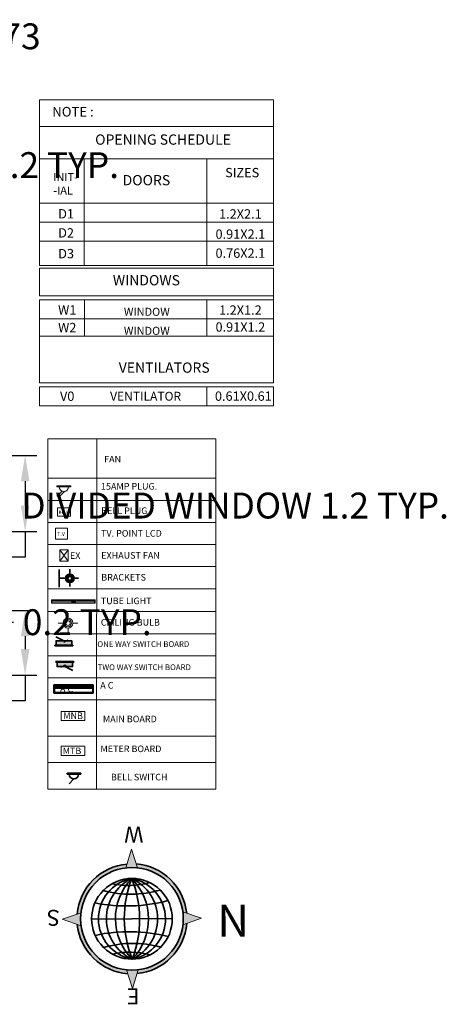
# Model space of a CAD drawing. Units: metres. Extents: x 24.2 to 58.5, y -14.5 to 15.2.
# Tile 7 of 7: x 51.9 to 58.5, y 0 to 15.2. Entities that reach past the tile are written whole.
import ezdxf

# ---------------------------------------------------------------- set-up
doc = ezdxf.new("R2010")
doc.units = ezdxf.units.M
doc.header["$MEASUREMENT"] = 0
for name, color, linetype, lineweight in [('A -Elec', 6, 'Continuous', 18), ('A- WALL', 7, 'Continuous', 35), ('A-ANNO-SCHD', 10, 'Continuous', 13), ('A-ANNO-SYMB', 90, 'Continuous', 18), ('A-ANNO-TEXT', 10, 'Continuous', 18), ('A-TEXT', 7, 'Continuous', 9), ('DIM', 7, 'Continuous', 9), ('DIMENSION', 90, 'Continuous', 18), ('E-ANNO-LEGN', 7, 'Continuous', 13), ('E-ANNO-TEXT', 7, 'Continuous', 18), ('E-COMM', 1, 'Continuous', 18), ('E-LITE', 1, 'Continuous', 18), ('E-POWR', 1, 'Continuous', 18), ('E-POWR-EQPM', 1, 'Continuous', 18), ('Elec', 1, 'Continuous', 35)]:
    doc.layers.add(name, color=color, linetype=linetype, lineweight=lineweight)
doc.styles.get("Standard").update_dxf_attribs({"font": 'arial.ttf'})
doc.dimstyles.get("Standard").update_dxf_attribs({"dimtxt": 0.4, "dimasz": 0.4, "dimexe": 0.18, "dimexo": 0.0625, "dimgap": 0.09, "dimtad": 0, "dimtih": 1, "dimtoh": 1, "dimdec": 1, "dimzin": 0, "dimdsep": 46, "dimtxsty": 'Standard', "dimcen": 0.09, "dimadec": 0, "dimazin": 0, "dimtfac": 1, "dimtdec": 1, "dimtofl": 0, "dimtmove": 0, "dimatfit": 3, "dimfxl": 1, "dimtolj": 1, "dimtzin": 0, "dimarcsym": 0})

# ---------------------------------------------------------------- blocks, each defined once
blk = doc.blocks.new('BELL SWITCH')
at = {"layer": 'Elec'}
for p, q in [((4981.810695824261, 3401.308516663301), (4981.810695824261, 3402.267205949833)), ((4981.810695824261, 3402.267205949833), (4993.567325880143, 3402.267205949833)), ((4993.567325880143, 3402.267205949833), (4993.567325880143, 3401.308516663301)), ((4993.567325880143, 3401.308516663301), (4981.810695824261, 3401.308516663301)), ((4987.689010852202, 3397.361748155474), (4983.521874140887, 3393.30038126191))]:
    blk.add_line(p, q, dxfattribs=at)
blk.add_arc((4987.689010852202, 3401.308516663301), 3.946768507828181, 180, 0, dxfattribs=at)
blk = doc.blocks.new('splight')
at = {"layer": 'Elec'}
for p, q in [((4618.165493646445, 527.1595508907546), (4627.57380882646, 527.1595508907546)), ((4622.869651236451, 527.1595508907546), (4622.869651236451, 523.8688723625129)), ((4620.576181531769, 521.5754026578305), (4618.052205676129, 521.5754026578305)), ((4622.869651236451, 519.2819329531479), (4622.869651236451, 517.0346704452847)), ((4625.163120941137, 521.5754026578305), (4627.232633020232, 521.5754026578305))]:
    blk.add_line(p, q, dxfattribs=at)
for radius in [2.293469704682637, 1.668469704682639, 1.043469704682639]:
    blk.add_circle((4622.869651236451, 521.5754026578305), radius, dxfattribs=at)
blk = doc.blocks.new('CIELING')
at = {"layer": 'A -Elec'}
for p, q in [((1070.869500591183, -8395.655580837194), (1070.869500591183, -8391.485789029257)), ((1066.613971407157, -8399.911110021205), (1062.44417959922, -8399.911110021205)), ((1075.125029775208, -8399.911110021205), (1079.294821583145, -8399.911110021205)), ((1070.869500591183, -8408.33643101315), (1070.869500591183, -8404.166639205214))]:
    blk.add_line(p, q, dxfattribs=at)
for radius in [4.255529184009533, 3.095842734009534, 1.936156284009533]:
    blk.add_circle((1070.869500591183, -8399.911110021205), radius, dxfattribs=at)
blk = doc.blocks.new('tube')
at = {"layer": 'A -Elec'}
for p, q in [((4592.607752765609, 556.7543292074987), (4641.607752765609, 556.7543292074987)), ((4592.607752765609, 555.2543292074988), (4592.607752765609, 556.7543292074987)), ((4592.607752765609, 552.7543292074987), (4592.607752765609, 555.2543292074988)), ((4593.107752765609, 555.2543292074988), (4593.107752765609, 556.7543292074987)), ((4593.107752765609, 556.3299144522243), (4593.407752765609, 556.3299144522243)), ((4593.107752765609, 556.2104979518087), (4593.407752765609, 556.2104979518087)), ((4593.107752765609, 555.8060867251079), (4593.407752765609, 555.8060867251079)), ((4593.107752765609, 555.6866702246923), (4593.407752765609, 555.6866702246923)), ((4641.107752765608, 555.2543292074988), (4593.107752765609, 555.2543292074988)), ((4593.107752765609, 555.2543292074988), (4593.107752765609, 553.2543292074988)), ((4593.107752765609, 553.2543292074988), (4593.107752765609, 555.2543292074988)), ((4593.407752765609, 555.2543292074988), (4593.407752765609, 556.7543292074987)), ((4593.407752765609, 556.5043292074988), (4640.807752765609, 556.5043292074988)), ((4593.407752765609, 556.2543292074987), (4640.807752765609, 556.2543292074987)), ((4593.407752765609, 556.0043292074988), (4640.807752765609, 556.0043292074988)), ((4593.407752765609, 555.7543292074988), (4640.807752765609, 555.7543292074988)), ((4593.407752765609, 555.5043292074988), (4640.807752765609, 555.5043292074988)), ((4640.807752765609, 555.2543292074988), (4640.807752765609, 556.7543292074987)), ((4640.807752765609, 556.3299144522243), (4641.107752765608, 556.3299144522243)), ((4640.807752765609, 556.2104979518087), (4641.107752765608, 556.2104979518087)), ((4640.807752765609, 555.8060867251079), (4641.107752765608, 555.8060867251079)), ((4640.807752765609, 555.6866702246923), (4641.107752765608, 555.6866702246923)), ((4641.107752765608, 556.7543292074987), (4641.107752765608, 555.2543292074988)), ((4641.107752765608, 555.2543292074988), (4641.107752765608, 556.7543292074987)), ((4641.107752765608, 553.2543292074988), (4641.107752765608, 555.2543292074988)), ((4641.607752765609, 556.7543292074987), (4641.607752765609, 555.2543292074988)), ((4641.607752765609, 552.7543292074987), (4641.607752765609, 555.2543292074988)), ((4592.607752765609, 552.7543292074987), (4641.607752765609, 552.7543292074987)), ((4593.107752765609, 553.2543292074988), (4641.607752765609, 553.2543292074988))]:
    blk.add_line(p, q, dxfattribs=at)
for points in [[(4615.603450108063, 553.2543292074988), (4619.112055423154, 553.2543292074988), (4619.112055423154, 554.3062122222327), (4615.603450108063, 554.3062122222327)], [(4619.112055423154, 553.7802707148657), (4619.112055423154, 553.7802707148657), (4619.112055423154, 553.7802707148657), (4619.112055423154, 553.7802707148657)], [(4619.112055423154, 553.7802707148657), (4619.813791770798, 553.7802707148657), (4619.813791770798, 553.2543292074988), (4619.112055423154, 553.2543292074988)]]:
    blk.add_lwpolyline(points, close=True, dxfattribs=at)
blk = doc.blocks.new('elec box')
at = {"layer": 'Elec'}
blk.add_hatch(color=256, dxfattribs=at).paths.add_polyline_path([(3828.234962737587, 599.2881263179643), (3828.234962737587, 594.7881263179643), (3844.734962737589, 594.7881263179643), (3844.734962737589, 599.2881263179643)])
for p, q in [((3836.484962737588, 599.2881263179643), (3828.066979685118, 603.4529863194257)), ((3846.10280273742, 594.7881263179643), (3826.830962060027, 594.7881263179643)), ((3826.830962060027, 594.7881263179643), (3826.830962060027, 593.8893551118417)), ((3826.830962060027, 593.8893551118417), (3846.10280273742, 593.8893551118417)), ((3846.10280273742, 593.8893551118417), (3846.10280273742, 594.7881263179643))]:
    blk.add_line(p, q, dxfattribs=at)
blk.add_lwpolyline([(3828.234962737587, 594.7881263179643), (3828.234962737587, 599.2881263179643), (3844.734962737589, 599.2881263179643), (3844.734962737589, 594.7881263179643), (3828.234962737587, 594.7881263179643)], dxfattribs=at)
blk = doc.blocks.new('DIRECTION')
at = {"layer": 'DIM', "ltscale": 35}
h = blk.add_hatch(color=256, dxfattribs=at)
h.dxf.hatch_style = 1
edge = h.paths.add_edge_path()
edge.add_line((2597.24832190935, 2408.269559539512), (2601.856533232682, 2393.62299110183))
edge.add_ellipse((2597.639423319343, 2353.481842285464), major_axis=(28.54028595385228, -28.5402859538523), ratio=0.9999999999827393, start_angle=129.0026750704451, end_angle=135.4089982327699)
edge.add_ellipse((2597.639423319602, 2353.481842285464), major_axis=(-28.54028595291803, -28.54028595291801), ratio=0.999999999985297, start_angle=225.4089982331304, end_angle=231.8159173823239)
edge.add_line((2592.849261358955, 2393.558645959323), (2597.248321909339, 2408.269559539583))
h = blk.add_hatch(color=256, dxfattribs=at)
h.dxf.hatch_style = 1
edge = h.paths.add_edge_path()
edge.add_line((2637.716337406115, 2348.692604170624), (2640.725786551334, 2349.752367405582))
edge.add_ellipse((2597.639423319343, 2353.481842285464), major_axis=(-30.58057945317442, -30.5805794531744), ratio=0.9999999999976388, start_angle=50.166226554127775, end_angle=130.0529151095595, ccw=False)
edge.add_line((2601.533664809112, 2310.41005845266), (2602.42916840349, 2313.404988786752))
edge.add_ellipse((2597.639423319343, 2353.481842285464), major_axis=(-28.54028595136435, -28.54028595136432), ratio=0.9999999999994514, start_angle=51.81532139532596, end_angle=128.185403391547)
edge = h.paths.add_edge_path()
edge.add_line((2593.421895860988, 2313.340737337358), (2594.360152675466, 2310.358877830749))
edge.add_ellipse((2597.639423319343, 2353.481842285464), major_axis=(-30.58057945314276, -30.58057945314273), ratio=0.9999999999967295, start_angle=320.7650813562228, end_angle=400.6513322142664, ccw=False)
edge.add_line((2554.610693956437, 2349.137635932355), (2557.634965847779, 2348.12094433685))
edge.add_ellipse((2597.639423319343, 2353.481842285464), major_axis=(28.54028595137265, -28.54028595137269), ratio=0.9999999999998977, start_angle=232.6325930742551, end_angle=309.0020790836279)
edge = h.paths.add_edge_path()
edge.add_line((2557.562509232831, 2358.271080400352), (2554.553060087694, 2357.211317165394))
edge.add_ellipse((2597.639423319343, 2353.481842285464), major_axis=(-30.58057945310715, -30.58057945310715), ratio=0.9999999999999497, start_angle=230.1666642515818, end_angle=310.0529151095499, ccw=False)
edge.add_line((2593.744852793148, 2396.553596367937), (2592.849261358943, 2393.558645959394))
edge.add_ellipse((2597.639423319343, 2353.481842285464), major_axis=(28.5402859513619, -28.54028595136188), ratio=0.9999999999987931, start_angle=141.8159173820852, end_angle=218.1854033915469)
edge = h.paths.add_edge_path()
edge.add_line((2601.85653323267, 2393.622991101876), (2600.918364535997, 2396.604831790109))
edge.add_ellipse((2597.639423319343, 2353.481842285464), major_axis=(-30.58057945312165, -30.58057945312163), ratio=0.9999999999985156, start_angle=140.765081356223, end_angle=220.6517699116423, ccw=False)
edge.add_line((2640.668152682508, 2357.826048638621), (2637.643880791167, 2358.842740234127))
edge.add_ellipse((2597.639423319343, 2353.481842285464), major_axis=(28.54028595137743, -28.54028595137745), ratio=0.9999999999999049, start_angle=52.63259307425506, end_angle=129.0026750705646)
h = blk.add_hatch(color=256, dxfattribs=at)
h.dxf.hatch_style = 1
edge = h.paths.add_edge_path()
edge.add_ellipse((2597.639423319343, 2353.481842285464), major_axis=(-28.54028595210723, -28.54028595210721), ratio=0.999999999994473, start_angle=308.1854033915466, end_angle=322.6325930742547)
edge.add_line((2557.634965847779, 2348.120944336826), (2542.851706063651, 2353.090740875343))
edge.add_line((2542.851706063651, 2353.090740875343), (2557.562509232831, 2358.271080400328))
h = blk.add_hatch(color=256, dxfattribs=at)
h.dxf.hatch_style = 1
edge = h.paths.add_edge_path()
edge.add_line((2637.643880791167, 2358.84274023415), (2652.427140575295, 2353.87294369554))
edge.add_line((2652.427140575295, 2353.87294369554), (2637.716337406114, 2348.692604170648))
edge.add_ellipse((2597.639423319343, 2353.481842285464), major_axis=(-28.54028595030189, -28.54028595030183), ratio=0.9999999999925798, start_angle=128.1854033915468, end_angle=142.632593074255)
h = blk.add_hatch(color=256, dxfattribs=at)
h.dxf.hatch_style = 1
edge = h.paths.add_edge_path()
edge.add_line((2602.42916840349, 2313.404988786869), (2598.030524729594, 2298.694125031464))
edge.add_line((2598.030524729594, 2298.69412503137), (2593.421895860988, 2313.340737337334))
edge.add_ellipse((2597.639423319602, 2353.481842285464), major_axis=(28.54028595190623, -28.54028595190623), ratio=0.9999999999939888, start_angle=-50.99792091661058, end_angle=-44.59100176735014)
edge.add_ellipse((2597.639423319343, 2353.481842285464), major_axis=(-28.54028595335771, -28.54028595335769), ratio=0.9999999999832972, start_angle=45.40899823301023, end_angle=51.81532139544526)
at = {"layer": 'A- WALL', "ltscale": 35}
blk.add_line((2629.34444276032, 2353.708168156072), (2565.934403878626, 2353.255516414717), dxfattribs=at)
at = {"layer": 'A- WALL', "ltscale": 35, "extrusion": (0, 0, -1)}
for centre, major_axis, ratio, start_param, end_param in [((2597.639423319343, 2353.481842285418), (-30.58057945312132, -30.58057945312131), 0.9999999999987959, 0.8717410831091346, 2.266019187658509), ((2597.639423319343, 2353.481842285418), (28.5402859514277, -28.5402859514277), 0.9999999999973692, 3.919852451189786, 10.20303775836937), ((2597.639423319343, 2353.481842285418), (-30.58057945314268, -30.58057945314266), 0.9999999999988618, 2.432085421867908, 3.826371165679486), ((2597.639423319343, 2353.481842285418), (22.41940544614458, -22.41940544614459), 0.999999999999132, 3.919852451188904, 10.20303775836849), ((2603.542187591361, 2353.523989522555), (22.80466912504525, -22.80466912504527), 0.9999999999934116, 0.9623333078138184, 3.735775406983438), ((2612.505423052941, 2353.587989301701), (-24.76160024723522, -24.76160024723521), 0.9999999999992525, -0.3540869259178678, 1.910602987118144), ((2629.757673802409, 2353.71112763613), (-31.9131967420592, -31.91319674205919), 0.9999999999985343, -0.0006610730671919, 1.55718066820378), ((2678.031679859687, 2354.055802032412), (-61.10857846222063, -61.10857846222057), 0.999999999998412, 0.4026080436482158, 1.153909784551204), ((2517.246998575127, 2352.907900606915), (61.1085784622124, -61.10857846221246), 0.9999999999999429, 5.114997024032398, 5.866298764935286), ((2565.521005037576, 2353.252518252051), (-31.91319674206676, -31.91319674206674), 0.9999999999991755, 3.140929813589933, 4.698771554849301), ((2591.736490906592, 2353.439704278876), (-22.80466912498845, -22.80466912498845), 0.9999999999995747, 2.533131401603469, 5.306573500773075), ((2582.773255331945, 2353.375720337799), (-24.76160024727029, -24.76160024727029), 0.9999999999990459, 2.78750749467719, 5.052197407698938), ((2597.115156409695, 2454.394147896003), (-57.71452300102988, -57.71452300102983), 0.9999999999994852, -1.068719002289636, -0.5124677756952505), ((2599.782951195766, 2490.828885281749), (89.95633825820524, -89.95633825820524), 0.9999999999996148, 0.5732801118446276, 1.028726990569549), ((2597.639423319343, 2353.481842285418), (-30.58057945309982, -30.5805794530998), 0.9999999999997768, -0.7094995924610965, 0.6847785120890495), ((2601.743533004009, 2216.179397968859), (-89.95633825845869, -89.95633825845869), 0.9999999999989515, 2.098588931419211, 2.554035810148795), ((2597.639423319343, 2353.481842285418), (-30.58057945319512, -30.58057945319512), 0.9999999999962719, 4.013333736700001, 5.407619480506816), ((2600.498417980858, 2261.332926481243), (-46.62855256648622, -46.6285525664862), 0.9999999999990784, 2.096633230266009, 2.553724030937174)]:
    blk.add_ellipse(centre, major_axis=major_axis, ratio=ratio, start_param=start_param, end_param=end_param, dxfattribs=at)
at = {"layer": 'A- WALL', "ltscale": 35, "extrusion": (0, 0, -0.9999999999999998)}
for centre, major_axis, ratio, start_param, end_param in [((2599.182585971628, 2445.662182832683), (46.62855256632114, -46.62855256632116), 0.9999999999994293, 0.5735918910566035, 1.030682691728694), ((2598.555858798734, 2252.572336165166), (-57.71452300096218, -57.71452300096211), 0.9999999999999362, 2.068987370893696, 2.625238597487658)]:
    blk.add_ellipse(centre, major_axis=major_axis, ratio=ratio, start_param=start_param, end_param=end_param, dxfattribs=at)
at = {"layer": 'DIM', "ltscale": 35}
for p, q in [((2597.24832190935, 2408.269559539489), (2592.827539238222, 2393.486004940269)), ((2597.24832190935, 2408.269559539489), (2601.879338537261, 2393.550507565663)), ((2542.851706063651, 2353.090740875319), (2557.656003696302, 2358.30400403195)), ((2542.851706063651, 2353.090740875319), (2557.728920809025, 2348.089358810546)), ((2652.427140575295, 2353.872943695493), (2637.549925830003, 2358.874325760384)), ((2652.427140575295, 2353.872943695493), (2637.622842942642, 2348.659680538956)), ((2598.030524729594, 2298.694125031323), (2602.450936591041, 2313.477790510296)), ((2598.030524729594, 2298.694125031323), (2593.399138912629, 2313.41306084311))]:
    blk.add_line(p, q, dxfattribs=at)
at = {"layer": 'A-TEXT', "char_height": 13.629465702112, "width": 273.2349075094469, "attachment_point": 2}
for s, insert in [('{\\fTimes New Roman|b0|i0|c0|p18;\\H0.9233x;E}', (2596.77738151443, 2420.65579489876)), ('{\\fTimes New Roman|b0|i0|c0|p18;\\H0.9233x;S}', (2659.361945474433, 2358.999040747372)), ('{\\fTimes New Roman|b0|i0|c0|p18;\\H0.9233x;W}', (2596.170612003199, 2293.619718441945))]:
    blk.add_mtext(s, dxfattribs=dict(at, insert=insert))
at = {"layer": 'A-TEXT', "insert": (2518.058106811495, 2342.398918831673), "char_height": 27.25893140422401, "width": 546.4698150188938, "attachment_point": 2, "rotation": 179.99999999999997}
blk.add_mtext('{\\fTimes New Roman|b0|i0|c0|p18;\\H0.9233x;N}', dxfattribs=at)
blk = doc.blocks.new('BELL-PLUG-POINT')
blk.add_lwpolyline([(-0.0004770172998647, 0.1300517861764519), (0.1983592237925009, 0.1300517861764519), (0.1983592237925009, 0.00049886287034), (-0.0004770172998647, 0.00049886287034)], close=True)
at = {"insert": (0.0190509924166875, 0.0853577644895012), "char_height": 0.0466140796815383, "attachment_point": 1}
blk.add_mtext('BELL', dxfattribs=at)
blk = doc.blocks.new('TV-POINT')
blk.add_lwpolyline([(-0.0002544828097726, 0.1689940023487439), (0.1847365432301089, 0.1689940023487439), (0.1847365432301089, 0.0001512106660435), (-0.0002544828097726, 0.0001512106660435)], close=True)
at = {"transparency": 33554676}
blk.add_lwpolyline([(-0.0002544828097726, 0.1689940023487439), (0.1847365432301089, 0.1689940023487439), (0.1847365432301089, 0.0001512106660435), (-0.0002544828097726, 0.0001512106660435)], close=True, dxfattribs=at)
at = {"insert": (0.0251958396718735, 0.110745502812601), "char_height": 0.0607508587558666, "attachment_point": 1}
blk.add_mtext('T.V ', dxfattribs=at)
at = {"transparency": 33554676, "insert": (0.0251958396718735, 0.110745502812601), "char_height": 0.0607508587558666, "attachment_point": 1}
blk.add_mtext('T.V ', dxfattribs=at)
blk = doc.blocks.new('METER-BOARD-TAG')
blk.add_lwpolyline([(0.000328818981032, 0.1428393106650341), (0.3660925782056239, 0.1428393106650341), (0.3660925782056239, 0.0002373866440166), (0.000328818981032, 0.0002373866440166)], close=True)
blk.add_text('MTB', height=0.101968299303365).set_placement((0.0267911737914091, 0.0212794313178835))
blk = doc.blocks.new('MAIN-BOARD-TAG')
blk.add_lwpolyline([(0.000328818981032, 0.1421226687325863), (0.3660925782056239, 0.1421226687325863), (0.3660925782056239, -0.0004792552884316), (0.000328818981032, -0.0004792552884316)], close=True)
blk.add_text('MNB', height=0.101968299303365).set_placement((0.0350054395535153, 0.0236772198803674))
blk = doc.blocks.new('SWITCHBOARD-ONE-WAY')
blk.add_line((0.1401166866044718, 0.0521100423505425), (0.2010258532319113, 0.0944184498532304))
at = {"xscale": 0.0145668999005024, "yscale": 0.0145668999005024, "zscale": 0.0145668999005024}
blk.add_blockref('elec box', (-55.74548794411445, -8.651445651998161), dxfattribs=at)
blk = doc.blocks.new('ac')
at = {"layer": 'Elec'}
for p, q in [((12718.33512872629, -53.78451556294852), (12674.35721837807, -53.78451556294852)), ((12674.35721837806, -63.01930683579224), (12674.35721837807, -53.78451556294852)), ((12675.81311487755, -57.52248662285011), (12675.81311487755, -53.78451556294851)), ((12717.02869991749, -54.85019267976269), (12675.81311487755, -54.85019267976269)), ((12717.02869991748, -57.52248662285011), (12717.02869991749, -53.78451556294851)), ((12718.33512872629, -63.01930683579224), (12718.33512872629, -53.78451556294852)), ((12718.33512872629, -63.01930683579224), (12674.35721837806, -63.01930683579224)), ((12674.88506837807, -57.52248662285011), (12717.80727872628, -57.52248662285011)), ((12717.02869991749, -56.20859049643797), (12675.81311487755, -56.20859049643797))]:
    blk.add_line(p, q, dxfattribs=at)
at = {"layer": 'Elec', "ltscale": 0.1}
for p, q in [((12674.88506837807, -61.49145683579366), (12674.88506837807, -53.78451556294851)), ((12717.02869991749, -54.35872395628861), (12675.81311487755, -54.35872395628861)), ((12717.80727872628, -61.49145683579366), (12717.80727872628, -53.78451556294851)), ((12717.02869991749, -55.65507023101156), (12675.81311487755, -55.65507023101157)), ((12717.02869991749, -56.84485043173038), (12675.81311487755, -56.84485043173037)), ((12716.80727872628, -62.49145683579365), (12675.88506837807, -62.49145683579365))]:
    blk.add_line(p, q, dxfattribs=at)
at = {"layer": 'Elec'}
for centre, start, end in [((12675.88506837807, -61.49145683579366), 180, 270), ((12716.80727872628, -61.49145683579366), 270, 0)]:
    blk.add_arc(centre, 1, start, end, dxfattribs=at)
blk = doc.blocks.new('AC-POINT-LABELED')
at = {"xscale": 0.0137983327653967, "yscale": 0.0137983327653967, "zscale": 0.0137983327653967}
blk.add_blockref('ac', (-174.8849808659187, 0.8696632936708708), dxfattribs=at)
blk.add_text(' A C', height=0.101968299303365).set_placement((0.0624941234119376, 0.0143010128270609))
blk = doc.blocks.new('*D59')
at = {"layer": 'Defpoints', "color": 0, "transparency": 16777216}
for p in [(48.22788193924818, 12.52982398857503), (48.4078819392482, 12.52982398857503), (48.22788193924818, 11.32982398857503)]:
    blk.add_point(p, dxfattribs=at)
at = {"layer": 'DIMENSION', "color": 0, "lineweight": -2, "transparency": 16777216}
for p, q in [((48.4078819392482, 12.52982398857503), (48.4078819392482, 12.92982398857503)), ((48.4078819392482, 12.92982398857503), (48.8078819392482, 12.92982398857503)), ((48.29038193924818, 12.52982398857503), (48.5878819392482, 12.52982398857503)), ((48.4078819392482, 11.72982398857503), (48.4078819392482, 12.12982398857503)), ((48.29038193924818, 11.32982398857503), (48.5878819392482, 11.32982398857503))]:
    blk.add_line(p, q, dxfattribs=at)
at = {"layer": 'DIMENSION', "color": 0, "transparency": 16777216}
for points in [[(48.34121527258154, 12.12982398857503), (48.47454860591487, 12.12982398857503), (48.4078819392482, 12.52982398857503)], [(48.34121527258154, 11.72982398857503), (48.47454860591487, 11.72982398857503), (48.4078819392482, 11.32982398857503)]]:
    blk.add_solid(points, dxfattribs=at)
at = {"layer": 'DIMENSION', "color": 0, "transparency": 16777216, "insert": (51.26077416298625, 12.92982398857502), "char_height": 0.4, "attachment_point": 5}
blk.add_mtext('\\A1;WINDOW 1.2 TYP.', dxfattribs=at)
blk = doc.blocks.new('*D63')
at = {"layer": 'Defpoints', "color": 0, "transparency": 16777216}
for p in [(51.03268193924821, 7.268149963184116), (51.21568193924823, 7.268149963184116), (51.03268193924821, 6.048149963184116)]:
    blk.add_point(p, dxfattribs=at)
at = {"layer": 'DIMENSION', "color": 0, "lineweight": -2, "transparency": 16777216}
for p, q in [((51.21568193924823, 7.268149963184116), (51.21568193924823, 7.668149963184117)), ((51.21568193924823, 7.668149963184117), (51.61568193924823, 7.668149963184117)), ((51.0951819392482, 7.268149963184116), (51.39568193924823, 7.268149963184116)), ((51.21568193924823, 6.448149963184116), (51.21568193924823, 6.868149963184116)), ((51.0951819392482, 6.048149963184116), (51.39568193924823, 6.048149963184116))]:
    blk.add_line(p, q, dxfattribs=at)
at = {"layer": 'DIMENSION', "color": 0, "transparency": 16777216}
for points in [[(51.14901527258156, 6.868149963184116), (51.2823486059149, 6.868149963184116), (51.21568193924823, 7.268149963184116)], [(51.14901527258156, 6.448149963184116), (51.2823486059149, 6.448149963184116), (51.21568193924823, 6.048149963184116)]]:
    blk.add_solid(points, dxfattribs=at)
at = {"layer": 'DIMENSION', "color": 0, "transparency": 16777216, "insert": (55.26134360364112, 7.6681499631841), "char_height": 0.4, "attachment_point": 5}
blk.add_mtext('\\A1;DIVIDED WINDOW 1.2 TYP.', dxfattribs=at)
blk = doc.blocks.new('*D64')
at = {"layer": 'Defpoints', "color": 0, "transparency": 16777216}
for p in [(50.88025193924815, 6.048149963184112), (51.03268193924818, 6.048149963184112), (51.03268193924818, 5.865149963184112)]:
    blk.add_point(p, dxfattribs=at)
at = {"layer": 'DIMENSION', "color": 0, "lineweight": -2, "transparency": 16777216}
for p, q in [((50.88025193924815, 5.985649963184112), (50.88025193924815, 5.685149963184112)), ((51.03268193924818, 5.985649963184112), (51.03268193924818, 5.685149963184112)), ((50.48025193924815, 5.865149963184112), (50.08025193924815, 5.865149963184112)), ((51.43268193924818, 5.865149963184112), (51.83268193924817, 5.865149963184112))]:
    blk.add_line(p, q, dxfattribs=at)
at = {"layer": 'DIMENSION', "color": 0, "transparency": 16777216}
for points in [[(50.48025193924815, 5.931816629850779), (50.48025193924815, 5.798483296517446), (50.88025193924815, 5.865149963184112)], [(51.43268193924818, 5.931816629850779), (51.43268193924818, 5.798483296517446), (51.03268193924818, 5.865149963184112)]]:
    blk.add_solid(points, dxfattribs=at)
at = {"layer": 'DIMENSION', "color": 0, "transparency": 16777216, "insert": (52.97384155725636, 5.865149963184112), "char_height": 0.4, "attachment_point": 5}
blk.add_mtext('\\A1;0.2 TYP.', dxfattribs=at)
blk = doc.blocks.new('*D113')
at = {"layer": 'Defpoints', "color": 0, "transparency": 16777216}
for p in [(51.03268200000003, 6.048150000000003), (51.03268200000003, 5.048824000000001), (52.01318200000006, 5.048824000000001)]:
    blk.add_point(p, dxfattribs=at)
at = {"layer": 'DIMENSION', "color": 0, "lineweight": -2, "transparency": 16777216}
for p, q in [((51.09518200000003, 6.048150000000003), (52.19318200000006, 6.048150000000003)), ((52.01318200000006, 5.648150000000002), (52.01318200000006, 5.448824000000001)), ((51.09518200000003, 5.048824000000001), (52.19318200000006, 5.048824000000001)), ((52.01318200000006, 5.048824000000001), (52.01318200000006, 4.648824000000001)), ((52.01318200000006, 4.648824000000001), (51.61318200000006, 4.648824000000001))]:
    blk.add_line(p, q, dxfattribs=at)
at = {"layer": 'DIMENSION', "color": 0, "transparency": 16777216}
for points in [[(51.94651533333338, 5.648150000000002), (52.07984866666673, 5.648150000000002), (52.01318200000006, 6.048150000000003)], [(51.94651533333338, 5.448824000000001), (52.07984866666673, 5.448824000000001), (52.01318200000006, 5.048824000000001)]]:
    blk.add_solid(points, dxfattribs=at)
at = {"layer": 'DIMENSION', "color": 0, "transparency": 16777216, "insert": (51.02318200000004, 4.648823999999985), "char_height": 0.4, "attachment_point": 5}
blk.add_mtext('\\A1;1.00', dxfattribs=at)
blk = doc.blocks.new('*D114')
at = {"layer": 'Defpoints', "color": 0, "transparency": 16777216}
for p in [(51.03268200000003, 8.442938000000003), (51.03268200000003, 7.268150000000003), (52.01318200000006, 7.268150000000003)]:
    blk.add_point(p, dxfattribs=at)
at = {"layer": 'DIMENSION', "color": 0, "lineweight": -2, "transparency": 16777216}
for p, q in [((51.09518200000003, 8.442938000000003), (52.19318200000006, 8.442938000000005)), ((52.01318200000006, 8.042938000000005), (52.01318200000006, 7.668150000000004)), ((51.09518200000003, 7.268150000000003), (52.19318200000006, 7.268150000000003)), ((52.01318200000006, 7.268150000000003), (52.01318200000006, 6.868150000000003)), ((52.01318200000006, 6.868150000000003), (51.61318200000006, 6.868150000000003))]:
    blk.add_line(p, q, dxfattribs=at)
at = {"layer": 'DIMENSION', "color": 0, "transparency": 16777216}
for points in [[(51.94651533333338, 8.042938000000003), (52.07984866666673, 8.042938000000005), (52.01318200000006, 8.442938000000005)], [(51.94651533333338, 7.668150000000004), (52.07984866666673, 7.668150000000004), (52.01318200000006, 7.268150000000003)]]:
    blk.add_solid(points, dxfattribs=at)
at = {"layer": 'DIMENSION', "color": 0, "transparency": 16777216, "insert": (51.02249987175993, 6.868149999999986), "char_height": 0.4, "attachment_point": 5}
blk.add_mtext('\\A1;1.17', dxfattribs=at)
blk = doc.blocks.new('*D121')
at = {"layer": 'Defpoints', "color": 0, "transparency": 16777216}
for p in [(50.313295, 14.920568), (49.587764, 8.639064), (50.313295, 8.639064)]:
    blk.add_point(p, dxfattribs=at)
at = {"layer": 'DIMENSION', "color": 0, "lineweight": -2, "transparency": 16777216}
for p, q in [((49.587764, 8.701564), (49.587764, 15.100568)), ((50.313295, 8.701564), (50.313295, 15.100568)), ((49.187764, 14.920568), (48.787764, 14.920568)), ((50.713295, 14.920568), (51.113295, 14.920568))]:
    blk.add_line(p, q, dxfattribs=at)
at = {"layer": 'DIMENSION', "color": 0, "transparency": 16777216}
for points in [[(49.187764, 14.98723466666666), (49.187764, 14.85390133333333), (49.587764, 14.920568)], [(50.713295, 14.98723466666666), (50.713295, 14.85390133333333), (50.313295, 14.920568)]]:
    blk.add_solid(points, dxfattribs=at)
at = {"layer": 'DIMENSION', "color": 0, "transparency": 16777216, "insert": (51.72280386766711, 14.920568), "char_height": 0.4, "attachment_point": 5}
blk.add_mtext('\\A1;0.73', dxfattribs=at)

msp = doc.modelspace()

# ---------------------------------------------------------------- linework, layer by layer
at = {"layer": 'A-ANNO-SCHD'}
for p, q in [((52.23786696983532, 13.9400684340007), (52.23786696983532, 11.75340257940532)), ((52.23786696983831, 13.52427876204881), (55.85399573796085, 13.52427876204881)), ((52.23786696983532, 13.02542588208799), (55.85399573636632, 13.02542588208799)), ((52.92865980590834, 12.34191459270067), (52.92865980590834, 13.02542588208799)), ((54.82490998105618, 12.34191459270067), (54.82490998105618, 13.02542588208799)), ((52.23786696983532, 12.34191459270067), (55.85399573417738, 12.34191459270067)), ((52.92865980590834, 11.380851027414), (52.92865980590834, 12.34191459270067)), ((54.82490998105618, 11.380851027414), (54.82490998105618, 12.34191459270067)), ((52.23786696983532, 12.04765858605326), (55.85399573323932, 12.04765858605326)), ((52.23786696983532, 11.75340257940532), (55.85399573229828, 11.75340257940532)), ((52.23786696983532, 11.75340257940532), (52.23786696983532, 11.380851027414)), ((55.85399573229828, 11.380851027414), (55.85399573356236, 11.74384444814902)), ((52.23786696983532, 11.380851027414), (55.85399573229828, 11.380851027414)), ((55.85399573277962, 10.84660136683377), (55.85399573434504, 11.336344408991)), ((52.92919215835256, 10.28742662729932), (52.9296580733419, 10.84660136683377)), ((54.82490998800708, 10.28742662729932), (54.82490998800708, 10.84660136683377)), ((52.23886523726893, 10.55234536018584), (55.85499396090255, 10.55234536018584)), ((52.23786697678921, 10.28742662729932), (55.85399570042381, 10.28742662729932)), ((54.82490999333254, 9.210786736713542), (54.82490999333254, 9.505042743361491))]:
    msp.add_line(p, q, dxfattribs=at)
for points in [[(52.23786696983532, 13.9400684340007), (55.85399574496557, 13.9400684340007), (55.85399573356236, 11.74384444814902)], [(55.85399573297968, 10.90895898627643), (52.23786697678921, 10.90895898627643), (52.23786697678921, 11.336344408991), (55.85399573434504, 11.336344408991)], [(52.23786697678921, 10.28742662729932), (52.23786697678921, 10.84660136683377), (55.85399573277962, 10.84660136683377), (55.85399573108388, 10.28742662729932)], [(55.853995728358, 9.210786736713542), (52.23786698210793, 9.210786736713542), (52.23786698210793, 9.505042743361491), (55.85399573023716, 9.505042743361491)], [(55.85399573023716, 9.505042743361491), (55.85399572835507, 9.210786736713542), (52.3052804933579, 9.210786736713542)]]:
    msp.add_lwpolyline(points, dxfattribs=at)
msp.add_lwpolyline([(55.85399573043718, 9.567400362804149), (52.23786698210793, 9.567400362804149), (52.23786698116986, 10.28742662729932), (55.85399573108388, 10.28742662729932), (55.85399573043718, 9.567400362804149)], close=True, dxfattribs=at)
at = {"layer": 'E-ANNO-LEGN'}
for p, q in [((52.36507160328699, 3.284869971333528), (52.36507160328699, 8.698996000703087)), ((54.96021383701208, 8.698996000703087), (52.36507160328699, 8.698996000703087)), ((53.12247395911057, 8.698996000703087), (53.11814065620005, 3.284869971333528)), ((54.96021383701179, 3.284869971333528), (54.96021383701179, 8.698996000703087)), ((54.96021383701208, 8.089965253070975), (52.36507160328699, 8.089965253070975)), ((54.96021383701208, 8.089965253071478), (52.36507160328699, 8.089965253071478)), ((54.96021383701208, 7.74858185870694), (52.36507160328699, 7.74858185870694)), ((54.96021383701179, 7.407198464342903), (52.36507160328648, 7.407198464342903)), ((54.96021383701208, 7.065815069978365), (52.36507160328699, 7.065815069978365)), ((54.96021383701208, 6.724431675614336), (52.36507160328699, 6.724431675614336)), ((54.96021383701208, 6.3830482812503), (52.36507160328699, 6.3830482812503)), ((54.96021383701179, 6.02930944892546), (52.36507160328648, 6.02930944892546)), ((54.96021383701179, 5.687926054560922), (52.36507160328648, 5.687926054560922)), ((54.96021383701179, 5.346542660196888), (52.36507160328648, 5.346542660196888)), ((54.96021383701208, 5.005159265832356), (52.36507160328699, 5.005159265832356)), ((54.96021383701208, 4.663775871468319), (52.36507160328699, 4.663775871468319)), ((54.96021383701208, 4.105764841524276), (52.36507160328699, 4.105764841524276)), ((54.96021383701208, 3.695317406429149), (52.36507160328699, 3.695317406429149)), ((54.96021383701208, 3.284869971333519), (52.36507160328699, 3.284869971333519))]:
    msp.add_line(p, q, dxfattribs=at)
at = {"layer": 'E-POWR'}
for p, q in [((52.5059050700018, 7.974805596766656), (52.71997713649061, 7.974805596766656)), ((52.5059050700018, 7.957349183175904), (52.5059050700018, 7.974805596766656)), ((52.71997713649061, 7.957349183175904), (52.5059050700018, 7.957349183175904)), ((52.71997713649061, 7.974805596766656), (52.71997713649061, 7.957349183175904)), ((52.58437630997554, 7.891404786369263), (52.50242345470917, 7.811532049698234)), ((52.62376658505528, 7.885483955945875), (52.54788875587324, 7.811532049698234)), ((52.62685655414134, 5.206232588683338), (52.5659473875139, 5.163924181179636)), ((52.62685655397769, 5.206232588684347), (52.68748097810399, 5.163517168469873))]:
    msp.add_line(p, q, dxfattribs=at)
msp.add_arc((52.61294110324659, 7.957349183175904), 0.0718652272298784, 180, 0, dxfattribs=at)
at = {"layer": 'E-POWR-EQPM'}
for p, q in [((52.54739005369419, 6.983274334849643), (52.67849215279852, 6.808471536043571)), ((52.67849215279852, 6.983274334849643), (52.54739005369419, 6.808471536043571))]:
    msp.add_line(p, q, dxfattribs=at)
msp.add_lwpolyline([(52.67849215279852, 6.983274334849643), (52.54739005369419, 6.983274334849643), (52.54739005369419, 6.808471536043571), (52.67849215279852, 6.808471536043571)], close=True, dxfattribs=at)

# ---------------------------------------------------------------- block references
at = {"layer": 'A-ANNO-SYMB', "xscale": 0.0196685805855262, "yscale": 0.0196685805855262, "zscale": 0.0196685805855262, "rotation": 180}
msp.add_blockref('DIRECTION', (104.7576541107284, 47.57055619885941), dxfattribs=at)
at = {"layer": 'E-COMM'}
for name, p in [('BELL-PLUG-POINT', (52.514, 7.504999999999999)), ('TV-POINT', (52.484, 7.15))]:
    msp.add_blockref(name, p, dxfattribs=at)
at = {"layer": 'E-COMM', "xscale": 0.0182086248757497, "yscale": 0.0182086248757497, "zscale": 0.0182086248757497}
msp.add_blockref('BELL SWITCH', (-38.05088512333195, -58.41765514365192), dxfattribs=at)
at = {"layer": 'E-LITE', "xscale": -0.0291629336008972, "yscale": 0.0291629336008972, "zscale": 0.0291629336007624, "rotation": 89.99999999999976}
msp.add_blockref('splight', (67.91550371828572, 141.3599519613867), dxfattribs=at)
at = {"layer": 'E-LITE', "transparency": 33554676}
for name, p, xscale, yscale, zscale in [('tube', (-10.72939881273544, -1.443500066434964), 0.0137504178205401, 0.0137504178205401, 0.0137504178205401), ('CIELING', (33.41885650039748, 156.9066494015668), 0.0179829907752924, 0.0179829907752924, 0.0179829907752924)]:
    msp.add_blockref(name, p, dxfattribs=dict(at, xscale=xscale, yscale=yscale, zscale=zscale))
at = {"layer": 'E-POWR'}
for name, p in [('SWITCHBOARD-ONE-WAY', (52.473, 5.5)), ('MAIN-BOARD-TAG', (52.568, 4.344999999999999)), ('METER-BOARD-TAG', (52.568, 3.805))]:
    msp.add_blockref(name, p, dxfattribs=at)
at = {"layer": 'E-POWR', "xscale": 0.0145668999005024, "yscale": 0.0145668999005024, "zscale": 0.0145668999005024, "rotation": 180}
msp.add_blockref('elec box', (108.5124611847786, 13.90978828303204), dxfattribs=at)
at = {"layer": 'E-POWR-EQPM'}
msp.add_blockref('AC-POINT-LABELED', (52.459, 4.769999999999999), dxfattribs=at)

# ---------------------------------------------------------------- texts
at = {"layer": 'A-ANNO-TEXT'}
for s, insert, char_height, width, attachment_point in [('{\\fTimes New Roman|b0|i0|c0|p18;NOTE :}', (52.43348832338475, 13.82932788796573), 0.148651923305853, 3.684829088066988, 1), ('{\\fTimes New Roman|b0|i0|c0|p18;OPENING SCHEDULE}', (54.14640064760323, 13.32490796709971), 0.1585620515262433, 4.367408666073758, 5), ('{\\fTimes New Roman|b0|i0|c0|p18;INIT-\\P-IAL}', (52.44856245398747, 12.80591666217542), 0.1238766027548775, 0.4383716795026914, 1), ('{\\fTimes New Roman|b0|i0|c0|p18;\\H0.8x;SIZES}', (55.37057715269466, 12.88645033247827), 0.1805136284226288, 1.158155278888691, 2), ('{\\fTimes New Roman|b0|i0|c0|p18;DOORS}', (53.88908969948374, 12.69726155748507), 0.1585620515262433, 4.367408666073758, 5), ('{\\fTimes New Roman|b0|i0|c0|p18;\\H0.8x;D1}', (52.64678881199009, 12.17723090752843), 0.1805136284226288, 0.6185498041018431, 5), ('{\\fTimes New Roman|b0|i0|c0|p18;\\H0.8x;1.2X2.1}', (55.34245155794265, 12.17575096186876), 0.1805141163197077, 1.435465247854927, 5), ('{\\fTimes New Roman|b0|i0|c0|p18;\\H0.8x;D2}', (52.64678881199009, 11.88297490088021), 0.1805136284226288, 0.6185498041018431, 5), ('{\\fTimes New Roman|b0|i0|c0|p18;\\H0.8x;0.91X2.1}', (55.34245155794265, 11.86349315487883), 0.1805141163197077, 1.435465247854927, 5), ('{\\fTimes New Roman|b0|i0|c0|p18;\\H0.8x;D3}', (52.64678881199009, 11.5619294339929), 0.1805136284226288, 0.6185498041018431, 5), ('{\\fTimes New Roman|b0|i0|c0|p18;\\H0.8x;0.76X2.1}', (55.34245155794265, 11.56923714823142), 0.1805141163197077, 1.435465247854927, 5), ('{\\fTimes New Roman|b0|i0|c0|p18;WINDOWS }', (53.88908970643466, 11.15094257208005), 0.1585620515262433, 4.367408666073758, 5), ('{\\fTimes New Roman|b0|i0|c0|p18;\\H0.8x;W1}', (52.66456616413172, 10.69151282569044), 0.1805141163197077, 0.6185498041018431, 5), ('{\\fTimes New Roman|b0|i0|c0|p18; WINDOW}', (53.87678490137407, 10.66316552920532), 0.1238766027548775, 2.44127520998431, 5), ('{\\fTimes New Roman|b0|i0|c0|p18;\\H0.8x;1.2X1.2}', (55.34245155794265, 10.6894373216876), 0.1805141163197077, 1.435465247854927, 5), ('{\\fTimes New Roman|b0|i0|c0|p18;\\H0.8x;0.91X1.2}', (55.34245155794265, 10.4278978592453), 0.1805141163197077, 1.435465247854927, 5), ('{\\fTimes New Roman|b0|i0|c0|p18;\\H0.8x;W2}', (52.66456616413172, 10.41954294114697), 0.1805141163197077, 0.6185498041018431, 5), ('{\\fTimes New Roman|b0|i0|c0|p18; WINDOW}', (53.87678490137407, 10.36890952255792), 0.1238766027548775, 2.44127520998431, 5), ('{\\fTimes New Roman|b0|i0|c0|p18;VENTILATORS }', (54.16434845826788, 9.800447677373649), 0.1585620515262433, 4.367408666073758, 5), ('{\\fTimes New Roman|b0|i0|c0|p18;\\H0.8x;V0}', (52.66356790897359, 9.35791474003711), 0.1805136284226288, 0.6185498041018431, 5), ('{\\fTimes New Roman|b0|i0|c0|p18;VENTILATOR}', (53.87678490575763, 9.35791474003711), 0.1362642630303653, 2.44127520998431, 5), ('{\\fTimes New Roman|b0|i0|c0|p18;\\H0.8x;0.61X0.61}', (55.38824012675052, 9.359653900766872), 0.1805141163197077, 1.435465247854927, 5)]:
    msp.add_mtext(s, dxfattribs=dict(at, insert=insert, char_height=char_height, width=width, attachment_point=attachment_point))
at = {"layer": 'E-ANNO-TEXT'}
for s, height, p in [('FAN', 0.101968299303365, (53.23538590752878, 8.33450178921115)), ('15AMP PLUG.', 0.101968299303365, (53.18661888659244, 7.913836581397111)), ('BELL PLUG', 0.101968299303365, (53.18986894252702, 7.537488956140537)), ('TV. POINT LCD', 0.101968299303365, (53.18701910611676, 7.187573437534813)), ('EXHAUST FAN', 0.101968299303365, (53.18986210765794, 6.846809889741138)), ('BRACKETS', 0.101968299303365, (53.19035558516659, 6.508516746574688)), ('TUBE LIGHT', 0.101968299303365, (53.18416015654969, 6.144228080405988)), ('CEILING BULB', 0.101968299303365, (53.18404138172309, 5.811817805481436)), ('ONE WAY SWITCH BOARD', 0.0883453345164354, (53.12964905708247, 5.48334493935992)), ('TWO WAY SWITCH BOARD', 0.0883453345164354, (53.13463282259258, 5.125210278412722)), (' A C', 0.101968299303365, (53.14396483822076, 4.838543848373157)), ('MAIN BOARD', 0.101968299303365, (53.21613528144502, 4.31903565003436)), ('METER BOARD', 0.101968299303365, (53.17828473557674, 3.857318682366756)), ('BELL SWITCH', 0.101968299303365, (53.34024369032295, 3.420433931598775))]:
    msp.add_text(s, height=height, dxfattribs=at).set_placement(p)
at = {"layer": 'E-POWR-EQPM', "insert": (52.70655032969955, 6.946494320487381), "char_height": 0.101968299303365, "width": 0.1780251574576642, "attachment_point": 1}
msp.add_mtext('EX', dxfattribs=at)

# ---------------------------------------------------------------- dimensions: what is measured, and where the dimension line sits
at = {"layer": 'DIMENSION'}
dim = msp.add_linear_dim(base=(50.313295, 14.920568), p1=(49.587764, 8.639064), p2=(50.313295, 8.639064), dimstyle='Standard', override={"dimdec": 2, "dimlfac": 1, "dimrnd": 0, "dimzin": 0, "dimdsep": 46, "dimlunit": 2}, dxfattribs=at)
dim.commit()
dim.dimension.update_dxf_attribs({"geometry": '*D121', "text_midpoint": (51.72280386766711, 14.920568)})
for base, p1, p2, text, picture, middle in [((48.4078819392482, 12.52982398857503), (48.22788193924814, 11.32982398857503), (48.22788193924814, 12.52982398857503), 'WINDOW <> TYP.', '*D59', (51.26077416298625, 12.92982398857502)), ((51.21568193924823, 7.268149963184116), (51.03268193924818, 6.048149963184112), (51.03268193924818, 7.268149963184113), 'DIVIDED WINDOW <> TYP.', '*D63', (55.26134360364112, 7.6681499631841))]:
    dim = msp.add_linear_dim(base=base, p1=p1, p2=p2, angle=90, text=text, dimstyle='Standard', override={"dimdec": 1, "dimlfac": 1, "dimrnd": 0, "dimzin": 0, "dimdsep": 46, "dimlunit": 2}, dxfattribs=at)
    dim.commit()
    dim.dimension.update_dxf_attribs({"geometry": picture, "text_midpoint": middle})
for base, p1, p2, angle, picture, middle in [((52.01318200000006, 7.268150000000003), (51.032682, 8.442938), (51.032682, 7.26815), 269.9999999999993, '*D114', (51.02249987175993, 6.868149999999986)), ((52.01318200000006, 5.048824000000001), (51.032682, 6.048149999999999), (51.032682, 5.048823999999999), 269.9999999999984, '*D113', (51.02318200000004, 4.648823999999985))]:
    dim = msp.add_linear_dim(base=base, p1=p1, p2=p2, angle=angle, dimstyle='Standard', override={"dimdec": 2, "dimlfac": 1, "dimrnd": 0, "dimzin": 0, "dimdsep": 46, "dimlunit": 2}, dxfattribs=at)
    dim.commit()
    dim.dimension.update_dxf_attribs({"geometry": picture, "text_midpoint": middle})
dim = msp.add_linear_dim(base=(51.03268193924818, 5.865149963184112), p1=(50.88025193924815, 6.048149963184112), p2=(51.03268193924818, 6.048149963184112), text='<> TYP.', dimstyle='Standard', override={"dimdec": 1, "dimlfac": 1, "dimrnd": 0, "dimzin": 0, "dimdsep": 46, "dimlunit": 2}, dxfattribs=at)
dim.commit()
dim.dimension.update_dxf_attribs({"geometry": '*D64', "text_midpoint": (52.97384155725636, 5.865149963184112)})

doc.saveas('drawing.dxf')
